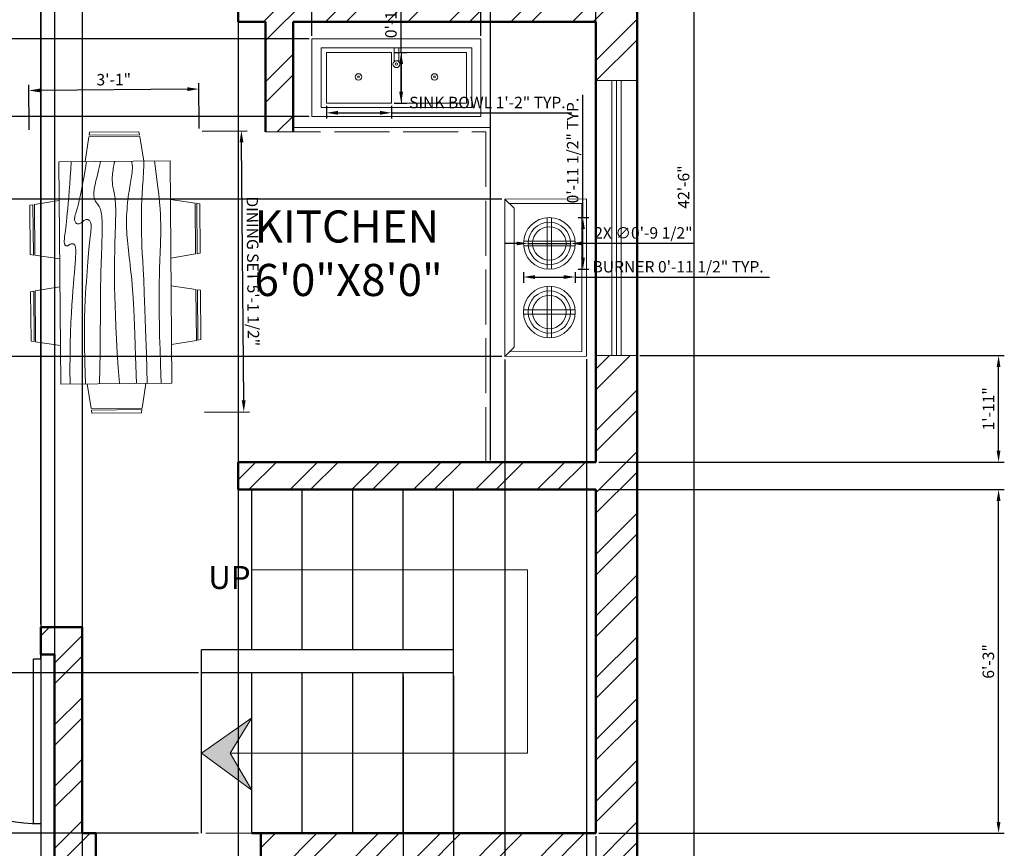
# Model space of a CAD drawing. Units: inches. Extents: x 1147 to 1568, y 1982 to 2559.
# Tile 3 of 4: x 1353 to 1568, y 2128 to 2309. Entities that reach past the tile are written whole.
import ezdxf

# ---------------------------------------------------------------- set-up
doc = ezdxf.new("R2010")
doc.units = ezdxf.units.IN
doc.linetypes.add('ACAD_ISO02W100', pattern=[15, 12, -3])
for name, color, linetype, lineweight in [('A-ANNO-DIMS', 2, 'Continuous', 18), ('A-ANNO-SYMB', 7, 'Continuous', 18), ('A-DOOR', 4, 'Continuous', 25), ('A-EQPM', 8, 'Continuous', 18), ('A-FLOR-CASE', 8, 'Continuous', 18), ('A-FLOR-CASE-HIDN', 8, 'ACAD_ISO02W100', 18), ('A-FLOR-FIXT', 8, 'Continuous', 18), ('A-FLOR-STRS', 7, 'Continuous', 25), ('A-WALL', 7, 'Continuous', 50), ('A-WALL-PATT', 252, 'Continuous', 13)]:
    doc.layers.add(name, color=color, linetype=linetype, lineweight=lineweight)
for name, color, linetype, lineweight, true_color in [('A-ANNO-TEXT', 244, 'Continuous', 18, 0x991b1e), ('A-AREA-IDEN', 244, 'Continuous', 25, 0x991b1e), ('A-FURN', 244, 'Continuous', 18, 0x991b1e), ('A-GLAZ', 177, 'Continuous', 18, 0x293189), ('A-WALL-OVHD', 244, 'ACAD_ISO02W100', 18, 0x991b1e)]:
    doc.layers.add(name, color=color, linetype=linetype, lineweight=lineweight, true_color=true_color)
doc.styles.get("Standard").update_dxf_attribs({"font": 'arial.ttf'})
doc.dimstyles.new('ISO-25', dxfattribs={"dimtxt": 2.5, "dimasz": 2.5, "dimexe": 1.25, "dimexo": 0.625, "dimtad": 1, "dimlunit": 3, "dimtxsty": 'Standard', "dimcen": 2.5, "dimadec": 0, "dimazin": 0, "dimtfac": 1, "dimtmove": 0, "dimatfit": 3, "dimfxl": 1, "dimarcsym": 0})

# ---------------------------------------------------------------- blocks, each defined once
blk = doc.blocks.new('*U3')
for p, q in [((-40, 0), (-40, 6)), ((0, 0), (0, 6))]:
    blk.add_line(p, q)
blk.add_lwpolyline([(0, 0), (0, -40), (-1.75, -40), (-1.75, 0)], close=True)
blk.add_arc((0, 0), 40, 180, 270)
blk = doc.blocks.new('Dining Set - 36 x 72 in.')
for p, q in [((-22.2343, 26.00059), (-23.4847, 17.99762)), ((-22.2304, 26), (-5.7608, 26)), ((-22, 27.5), (-22.1562, 26.50042)), ((-5.8416, 26.5), (-22.1534, 26.5)), ((-22, 27.5), (-6, 27.5)), ((-5.8437, 26.49966), (-6, 27.5)), ((-4.5152, 17.99762), (-5.7655, 25.99926)), ((5.7657, 26.00059), (4.5153, 17.99762)), ((5.7696, 26), (22.2392, 26)), ((6, 27.5), (5.8438, 26.50042)), ((22.1584, 26.5), (5.8466, 26.5)), ((6, 27.5), (22, 27.5)), ((22.1563, 26.49966), (22, 27.5)), ((23.4848, 17.99762), (22.2345, 25.99926)), ((36, 18), (-36, 18)), ((-36, 18), (-36, -18)), ((36, -18), (36, 18)), ((-45.5, 8), (-44.5004, 8.15617)), ((-45.5, 8), (-45.5, -8)), ((-44.5, -8.15843), (-44.5, 8.15338)), ((-44.0006, 8.23428), (-35.9976, 9.48474)), ((-44, 8.23041), (-44, -8.23915)), ((44.0006, 8.23428), (35.9976, 9.48474)), ((44, 8.23041), (44, -8.23915)), ((44.5, -8.15843), (44.5, 8.15338)), ((45.5, 8), (44.5005, 8.15617)), ((45.5, 8), (45.5, -8)), ((-44.4997, -8.15631), (-45.5, -8)), ((-35.9976, -9.48476), (-43.9993, -8.2345)), ((35.9976, -9.48476), (43.9993, -8.2345)), ((44.4997, -8.15631), (45.5, -8)), ((-36, -18), (36, -18)), ((-22.2343, -26.0006), (-23.4847, -17.99762)), ((-4.5152, -17.99762), (-5.7655, -25.99928)), ((5.7657, -26.0006), (4.5153, -17.99762)), ((23.4848, -17.99762), (22.2345, -25.99928)), ((-22.2304, -26), (-5.7608, -26)), ((-22, -27.5), (-22.1562, -26.50044)), ((-5.8416, -26.5), (-22.1534, -26.5)), ((-22, -27.5), (-6, -27.5)), ((-5.8437, -26.49967), (-6, -27.5)), ((5.7696, -26), (22.2392, -26)), ((6, -27.5), (5.8438, -26.50044)), ((22.1584, -26.5), (5.8466, -26.5)), ((6, -27.5), (22, -27.5)), ((22.1563, -26.49967), (22, -27.5))]:
    blk.add_line(p, q)
for points in [[(-36, 15), (-31.1772, 14.97754), (-26.8079, 14.91406), (-22.8538, 14.81543), (-19.276, 14.6875), (-16.0362, 14.53613), (-13.0957, 14.36718), (-10.4159, 14.18652), (-7.9583, 14), (-5.6904, 13.81315), (-3.6035, 13.63021), (-1.6954, 13.45508), (0.0365, 13.29166), (1.5945, 13.14388), (2.9811, 13.01562), (4.1988, 12.9108), (5.25, 12.83333), (6.1393, 12.78613), (6.8802, 12.76823), (7.4883, 12.77767), (7.9792, 12.8125), (8.3685, 12.87077), (8.6719, 12.95052), (8.9049, 13.0498), (9.0833, 13.16666), (9.2205, 13.29899), (9.3216, 13.44401), (9.3895, 13.59879), (9.4271, 13.76041), (9.4373, 13.92594), (9.4232, 14.09245), (9.3875, 14.257), (9.3333, 14.41666), (9.2638, 14.56917), (9.1836, 14.71484), (9.0975, 14.85465), (9.0104, 14.98958), (8.9272, 15.1206), (8.8529, 15.2487), (8.7922, 15.37483), (8.75, 15.5), (8.7305, 15.62467), (8.7344, 15.74739), (8.7617, 15.86621), (8.8125, 15.97916), (8.8867, 16.08431), (8.9844, 16.17968), (9.1055, 16.26334), (9.25, 16.33333), (9.4189, 16.38802), (9.6172, 16.42708), (9.8506, 16.45052), (10.125, 16.45833), (10.4463, 16.45052), (10.8203, 16.42708), (11.2529, 16.38802), (11.75, 16.33333), (12.3184, 16.26318), (12.9694, 16.17838), (13.7151, 16.07991), (14.5677, 15.96875), (15.5395, 15.84586), (16.6426, 15.71224), (17.8893, 15.56884), (19.2917, 15.41666), (20.859, 15.25667), (22.5879, 15.08984), (24.4721, 14.91715), (26.5052, 14.73958), (28.6809, 14.5581), (30.9929, 14.3737), (33.4347, 14.18733), (36, 14)], [(-36, 10), (-28.9766, 10.14274), (-23.1725, 10.20442), (-18.4241, 10.19775), (-14.5677, 10.13541), (-11.4399, 10.03011), (-8.877, 9.89453), (-6.7154, 9.74137), (-4.7917, 9.58333), (-2.9698, 9.43082), (-1.2246, 9.28515), (0.4415, 9.14534), (2.026, 9.01041), (3.5266, 8.87939), (4.9408, 8.7513), (6.266, 8.62516), (7.5, 8.5), (8.6411, 8.37549), (9.6914, 8.2539), (10.6538, 8.13818), (11.5312, 8.03125), (12.3267, 7.93603), (13.043, 7.85547), (13.6831, 7.79248), (14.25, 7.75), (14.7471, 7.7303), (15.1797, 7.73307), (15.5537, 7.75732), (15.875, 7.80208), (16.1494, 7.86637), (16.3828, 7.94922), (16.5811, 8.04964), (16.75, 8.16666), (16.8944, 8.29915), (17.0143, 8.44531), (17.1089, 8.60319), (17.1771, 8.77083), (17.218, 8.94629), (17.2305, 9.1276), (17.2137, 9.31282), (17.1667, 9.5), (17.0895, 9.6875), (16.987, 9.875), (16.8649, 10.0625), (16.7292, 10.25), (16.5856, 10.4375), (16.4401, 10.625), (16.2985, 10.8125), (16.1667, 11), (16.05, 11.18733), (15.9518, 11.3737), (15.8752, 11.5581), (15.8229, 11.73958), (15.798, 11.91715), (15.8034, 12.08984), (15.842, 12.25667), (15.9167, 12.41666), (16.0295, 12.56836), (16.1784, 12.70833), (16.3605, 12.83268), (16.5729, 12.9375), (16.8127, 13.01888), (17.0768, 13.07291), (17.3625, 13.0957), (17.6667, 13.08333), (17.9894, 13.03312), (18.3418, 12.94726), (18.7382, 12.82918), (19.1927, 12.68229), (19.7195, 12.51001), (20.3327, 12.31575), (21.0465, 12.10294), (21.875, 11.875), (22.8357, 11.63354), (23.959, 11.37304), (25.2786, 11.08618), (26.8282, 10.76562), (28.6414, 10.40405), (30.752, 9.99414), (33.1936, 9.52856), (36, 9)], [(-36, 5.5), (-30.7157, 5.3348), (-26.069, 5.20963), (-21.9946, 5.11767), (-18.4271, 5.05208), (-15.3009, 5.00602), (-12.5508, 4.97265), (-10.1112, 4.94515), (-7.9167, 4.91666), (-5.909, 4.88167), (-4.0586, 4.83984), (-2.3429, 4.79215), (-0.7396, 4.73958), (0.7739, 4.6831), (2.22, 4.6237), (3.6213, 4.56233), (5, 4.5), (6.373, 4.43782), (7.7344, 4.3776), (9.0723, 4.32129), (10.375, 4.27083), (11.6309, 4.22819), (12.8281, 4.19531), (13.9551, 4.17415), (15, 4.16666), (15.954, 4.17448), (16.819, 4.19791), (17.6001, 4.23698), (18.3021, 4.29166), (18.9299, 4.36198), (19.4883, 4.44791), (19.9823, 4.54948), (20.4167, 4.66666), (20.7969, 4.79899), (21.1302, 4.94401), (21.4245, 5.09879), (21.6875, 5.26041), (21.9271, 5.42594), (22.1511, 5.59245), (22.3672, 5.757), (22.5834, 5.91666), (22.8065, 6.06868), (23.0404, 6.21093), (23.2879, 6.34147), (23.5521, 6.45833), (23.8358, 6.55957), (24.142, 6.64323), (24.4735, 6.70735), (24.8334, 6.75), (25.2235, 6.76969), (25.642, 6.76692), (26.0858, 6.74267), (26.5521, 6.69791), (27.0379, 6.63362), (27.5404, 6.55078), (28.0565, 6.45036), (28.5834, 6.33333), (29.1242, 6.19987), (29.7071, 6.04687), (30.3661, 5.87044), (31.1354, 5.66666), (32.0493, 5.43164), (33.142, 5.16146), (34.4475, 4.85221), (36, 4.5)], [(-36, -1), (-30.7915, -0.6591), (-26.0195, -0.38216), (-21.6519, -0.16284), (-17.6563, 0.00521), (-14.0005, 0.12833), (-10.6523, 0.21289), (-7.5796, 0.26522), (-4.75, 0.29166), (-2.134, 0.29793), (0.2878, 0.28711), (2.5317, 0.26163), (4.6146, 0.22396), (6.5529, 0.17651), (8.3633, 0.12174), (10.0623, 0.06209), (11.6667, 0), (13.1899, -0.06201), (14.6341, -0.1211), (15.9982, -0.17432), (17.2813, -0.21875), (18.4823, -0.25147), (19.6003, -0.26953), (20.6343, -0.27002), (21.5834, -0.25), (22.4481, -0.20768), (23.2357, -0.14584), (23.9549, -0.06836), (24.6146, 0.02083), (25.2235, 0.11784), (25.7904, 0.21875), (26.3241, 0.31966), (26.8334, 0.41666), (27.3265, 0.50618), (27.8099, 0.58593), (28.2894, 0.65397), (28.7709, 0.70833), (29.2601, 0.74707), (29.763, 0.76823), (30.2855, 0.76985), (30.8334, 0.75), (31.4088, 0.70784), (31.9994, 0.64713), (32.589, 0.57275), (33.1615, 0.48958), (33.7008, 0.4025), (34.1908, 0.3164), (34.6153, 0.23616), (34.9584, 0.16666), (35.2099, 0.11165), (35.3848, 0.07031), (35.504, 0.04069), (35.5886, 0.02083), (35.6594, 0.00879), (35.7377, 0.0026), (35.8442, 0.00032), (36, 0)], [(-36, -6.5), (-27.1843, -6.31267), (-20.084, -6.1263), (-14.469, -5.9419), (-10.1094, -5.76042), (-6.7752, -5.58285), (-4.2363, -5.41016), (-2.2629, -5.24333), (-0.625, -5.08334), (0.8708, -4.93099), (2.2715, -4.78646), (3.5872, -4.64974), (4.8281, -4.52084), (6.0046, -4.39974), (7.127, -4.28646), (8.2053, -4.18099), (9.25, -4.08334), (10.2705, -3.99382), (11.2734, -3.91407), (12.2647, -3.84603), (13.25, -3.79167), (14.2354, -3.75293), (15.2266, -3.73177), (16.2295, -3.73015), (17.25, -3.75), (18.2912, -3.79248), (19.3451, -3.85547), (20.4009, -3.93604), (21.4479, -4.03125), (22.4754, -4.13819), (23.4727, -4.25391), (24.4289, -4.37549), (25.3334, -4.5), (26.1785, -4.62492), (26.9694, -4.74935), (27.7145, -4.87281), (28.4219, -4.99479), (29.1, -5.11483), (29.7572, -5.23242), (30.4016, -5.34709), (31.0417, -5.45834), (31.6837, -5.56437), (32.3262, -5.65821), (32.9658, -5.73153), (33.599, -5.77604), (34.2224, -5.78345), (34.8327, -5.74545), (35.4264, -5.65373), (36, -5.5)], [(-36, -10), (-26.4022, -9.81299), (-18.4675, -9.62891), (-11.9839, -9.45069), (-6.7396, -9.28125), (-2.5226, -9.12354), (0.8789, -8.98047), (3.6769, -8.85498), (6.0833, -8.75), (8.2767, -8.66765), (10.3021, -8.60677), (12.1712, -8.56543), (13.8958, -8.54167), (15.4876, -8.53353), (16.9583, -8.53907), (18.3197, -8.55632), (19.5834, -8.58334), (20.7616, -8.61841), (21.8685, -8.66081), (22.9188, -8.71004), (23.9271, -8.76563), (24.9081, -8.82707), (25.8763, -8.89388), (26.8465, -8.96558), (27.8334, -9.04167), (28.8474, -9.12118), (29.8828, -9.20117), (30.93, -9.27824), (31.9792, -9.34896), (33.0205, -9.40991), (34.0443, -9.45768), (35.0407, -9.48885), (36, -9.5)], [(-36, -14.5), (-30.0881, -14.33513), (-25.0332, -14.21224), (-20.7312, -14.12647), (-17.0781, -14.07292), (-13.97, -14.04671), (-11.3027, -14.04297), (-8.9724, -14.05681), (-6.875, -14.08334), (-4.9224, -14.11833), (-3.0905, -14.16016), (-1.3709, -14.20785), (0.2448, -14.26042), (1.7647, -14.3169), (3.1973, -14.3763), (4.5507, -14.43767), (5.8333, -14.5), (7.0554, -14.5621), (8.235, -14.62175), (9.3922, -14.67652), (10.5469, -14.72396), (11.7192, -14.76164), (12.929, -14.78711), (14.1965, -14.79794), (15.5417, -14.79167), (16.9933, -14.76424), (18.6152, -14.70508), (20.4804, -14.60197), (22.6615, -14.44271), (25.2312, -14.21509), (28.2624, -13.9069), (31.8277, -13.50594), (36, -13)]]:
    blk.add_lwpolyline(points)
blk = doc.blocks.new('*D13')
at = {"layer": 'A-ANNO-DIMS', "color": 0, "lineweight": -2, "transparency": 16777216}
for p, q in [((1488.23, 2527.7), (1501.22, 2527.7)), ((1499.97, 2525.2), (1499.97, 2020.2)), ((1488.23, 2017.7), (1501.22, 2017.7))]:
    blk.add_line(p, q, dxfattribs=at)
at = {"layer": 'A-ANNO-DIMS', "color": 0, "transparency": 16777216}
for points in [[(1499.56, 2525.2), (1500.39, 2525.2), (1499.97, 2527.7)], [(1499.56, 2020.2), (1500.39, 2020.2), (1499.97, 2017.7)]]:
    blk.add_solid(points, dxfattribs=at)
at = {"layer": 'Defpoints', "color": 0, "transparency": 16777216}
for p in [(1487.61, 2527.7), (1487.61, 2017.7), (1499.97, 2017.7)]:
    blk.add_point(p, dxfattribs=at)
at = {"layer": 'A-ANNO-DIMS', "color": 0, "transparency": 16777216, "insert": (1498.07, 2272.7), "char_height": 2.5, "attachment_point": 5, "rotation": 90}
blk.add_mtext('42\'-6"', dxfattribs=at)
blk = doc.blocks.new('WIN-GLAZ-60IN')
for p, q in [((0, 60), (0, 0)), ((1, 60), (1, 0)), ((2, 60), (2, 0))]:
    blk.add_line(p, q)
blk = doc.blocks.new('COOKTOP-BURNER')
for p, q in [((5.14, 11.27), (5.14, 0)), ((6.14, 11.27), (6.14, 0)), ((0, 6.14), (11.27, 6.14)), ((0, 5.14), (11.27, 5.14))]:
    blk.add_line(p, q)
for radius in [5.64, 4.64, 3.64]:
    blk.add_circle((5.64, 5.64), radius)
blk = doc.blocks.new('SINK-BOWL-WITH-DRAIN')
blk.add_lwpolyline([(0, 11.03), (14.13, 11.03), (14.13, 0), (0, 0)], close=True)
for radius in [0.702, 0.202]:
    blk.add_circle((6.95, 5.7), radius)
blk = doc.blocks.new('*D29')
at = {"layer": 'A-ANNO-DIMS', "color": 0, "lineweight": -2, "transparency": 16777216}
for p, q in [((1462.84, 2254.12), (1462.84, 2251.81)), ((1474.11, 2254.12), (1474.11, 2251.81)), ((1465.34, 2253.06), (1471.61, 2253.06)), ((1474.11, 2253.06), (1516.47, 2253.06))]:
    blk.add_line(p, q, dxfattribs=at)
at = {"layer": 'A-ANNO-DIMS', "color": 0, "transparency": 16777216}
for points in [[(1465.34, 2253.47), (1465.34, 2252.64), (1462.84, 2253.06)], [(1471.61, 2253.47), (1471.61, 2252.64), (1474.11, 2253.06)]]:
    blk.add_solid(points, dxfattribs=at)
at = {"layer": 'Defpoints', "color": 0, "transparency": 16777216}
for p in [(1462.84, 2254.75), (1474.11, 2254.75), (1474.11, 2253.06)]:
    blk.add_point(p, dxfattribs=at)
at = {"layer": 'A-ANNO-DIMS', "color": 0, "transparency": 16777216, "insert": (1496.54, 2254.98), "char_height": 2.5, "attachment_point": 5}
blk.add_mtext('BURNER 0\'-11 1/2" TYP.', dxfattribs=at)
blk = doc.blocks.new('*D30')
at = {"layer": 'A-ANNO-DIMS', "color": 0, "lineweight": -2, "transparency": 16777216}
for p, q in [((1475.8, 2266.02), (1475.8, 2292.78)), ((1474.73, 2266.02), (1477.05, 2266.02)), ((1475.8, 2257.25), (1475.8, 2263.52)), ((1474.73, 2254.75), (1477.05, 2254.75))]:
    blk.add_line(p, q, dxfattribs=at)
at = {"layer": 'A-ANNO-DIMS', "color": 0, "transparency": 16777216}
for points in [[(1475.38, 2263.52), (1476.22, 2263.52), (1475.8, 2266.02)], [(1475.38, 2257.25), (1476.22, 2257.25), (1475.8, 2254.75)]]:
    blk.add_solid(points, dxfattribs=at)
at = {"layer": 'Defpoints', "color": 0, "transparency": 16777216}
for p in [(1474.11, 2266.02), (1475.8, 2266.02), (1474.11, 2254.75)]:
    blk.add_point(p, dxfattribs=at)
at = {"layer": 'A-ANNO-DIMS', "color": 0, "transparency": 16777216, "insert": (1473.88, 2280.65), "char_height": 2.5, "attachment_point": 5, "rotation": 90}
blk.add_mtext('0\'-11 1/2" TYP.', dxfattribs=at)
blk = doc.blocks.new('*D31')
at = {"layer": 'A-ANNO-DIMS', "color": 0, "lineweight": -2, "transparency": 16777216}
for p, q in [((1419.91, 2290.39), (1419.91, 2287.64)), ((1434.04, 2290.39), (1434.04, 2287.64)), ((1422.41, 2288.89), (1431.54, 2288.89)), ((1434.04, 2288.89), (1473.4, 2288.89))]:
    blk.add_line(p, q, dxfattribs=at)
at = {"layer": 'A-ANNO-DIMS', "color": 0, "transparency": 16777216}
for points in [[(1422.41, 2289.31), (1422.41, 2288.47), (1419.91, 2288.89)], [(1431.54, 2289.31), (1431.54, 2288.47), (1434.04, 2288.89)]]:
    blk.add_solid(points, dxfattribs=at)
at = {"layer": 'Defpoints', "color": 0, "transparency": 16777216}
for p in [(1419.91, 2291.01), (1434.04, 2291.01), (1434.04, 2288.89)]:
    blk.add_point(p, dxfattribs=at)
at = {"layer": 'A-ANNO-DIMS', "color": 0, "transparency": 16777216, "insert": (1454.97, 2290.81), "char_height": 2.5, "attachment_point": 5}
blk.add_mtext('SINK BOWL 1\'-2" TYP.', dxfattribs=at)
blk = doc.blocks.new('*D32')
at = {"layer": 'A-ANNO-DIMS', "color": 0, "lineweight": -2, "transparency": 16777216}
for p, q in [((1436.16, 2302.04), (1436.16, 2322.97)), ((1434.67, 2302.04), (1437.41, 2302.04)), ((1436.16, 2293.51), (1436.16, 2299.54)), ((1434.67, 2291.01), (1437.41, 2291.01))]:
    blk.add_line(p, q, dxfattribs=at)
at = {"layer": 'A-ANNO-DIMS', "color": 0, "transparency": 16777216}
for points in [[(1435.75, 2299.54), (1436.58, 2299.54), (1436.16, 2302.04)], [(1435.75, 2293.51), (1436.58, 2293.51), (1436.16, 2291.01)]]:
    blk.add_solid(points, dxfattribs=at)
at = {"layer": 'Defpoints', "color": 0, "transparency": 16777216}
for p in [(1434.04, 2302.04), (1436.16, 2302.04), (1434.04, 2291.01)]:
    blk.add_point(p, dxfattribs=at)
at = {"layer": 'A-ANNO-DIMS', "color": 0, "transparency": 16777216, "insert": (1434.26, 2313.75), "char_height": 2.5, "attachment_point": 5, "rotation": 90}
blk.add_mtext('0\'-11" TYP.', dxfattribs=at)
blk = doc.blocks.new('*D37')
at = {"layer": 'A-ANNO-DIMS', "color": 0, "lineweight": -2, "transparency": 16777216}
for p, q in [((1392.77, 2284.88), (1402.59, 2284.96)), ((1401.84, 2226.14), (1401.36, 2282.45)), ((1393.29, 2223.57), (1403.11, 2223.65))]:
    blk.add_line(p, q, dxfattribs=at)
at = {"layer": 'A-ANNO-DIMS', "color": 0, "transparency": 16777216}
for points in [[(1401.78, 2282.45), (1400.94, 2282.44), (1401.34, 2284.95)], [(1402.26, 2226.15), (1401.42, 2226.14), (1401.86, 2223.64)]]:
    blk.add_solid(points, dxfattribs=at)
at = {"layer": 'Defpoints', "color": 0, "transparency": 16777216}
for p in [(1392.14, 2284.87), (1401.34, 2284.95), (1392.67, 2223.57)]:
    blk.add_point(p, dxfattribs=at)
at = {"layer": 'A-ANNO-DIMS', "color": 0, "transparency": 16777216, "insert": (1403.52, 2254.31), "char_height": 2.5, "attachment_point": 5, "rotation": 270.4889}
blk.add_mtext('DINING SET 5\'-1 1/2"', dxfattribs=at)
blk = doc.blocks.new('*D38')
at = {"layer": 'A-ANNO-DIMS', "color": 0, "lineweight": -2, "transparency": 16777216}
for p, q in [((1355.09, 2285.18), (1355, 2295)), ((1392.14, 2285.49), (1392.05, 2295.32)), ((1389.56, 2294.04), (1357.51, 2293.77))]:
    blk.add_line(p, q, dxfattribs=at)
at = {"layer": 'A-ANNO-DIMS', "color": 0, "transparency": 16777216}
for points in [[(1357.51, 2294.19), (1357.52, 2293.35), (1355.01, 2293.75)], [(1389.56, 2294.46), (1389.57, 2293.63), (1392.06, 2294.07)]]:
    blk.add_solid(points, dxfattribs=at)
at = {"layer": 'Defpoints', "color": 0, "transparency": 16777216}
for p in [(1355.01, 2293.75), (1355.09, 2284.55), (1392.14, 2284.87)]:
    blk.add_point(p, dxfattribs=at)
at = {"layer": 'A-ANNO-DIMS', "color": 0, "transparency": 16777216, "insert": (1373.52, 2295.81), "char_height": 2.5, "attachment_point": 5, "rotation": 0.4889}
blk.add_mtext('3\'-1"', dxfattribs=at)
blk = doc.blocks.new('*D43')
at = {"layer": 'A-ANNO-DIMS', "color": 0, "lineweight": -2, "transparency": 16777216}
for p, q in [((1327.61, 2368.08), (1327.61, 1981.52)), ((1357.61, 2368.08), (1357.61, 1981.52)), ((1330.11, 1982.77), (1355.11, 1982.77))]:
    blk.add_line(p, q, dxfattribs=at)
at = {"layer": 'A-ANNO-DIMS', "color": 0, "transparency": 16777216}
for points in [[(1330.11, 1983.19), (1330.11, 1982.35), (1327.61, 1982.77)], [(1355.11, 1983.19), (1355.11, 1982.35), (1357.61, 1982.77)]]:
    blk.add_solid(points, dxfattribs=at)
at = {"layer": 'Defpoints', "color": 0, "transparency": 16777216}
for p in [(1327.61, 2368.7), (1357.61, 2368.7), (1357.61, 1982.77)]:
    blk.add_point(p, dxfattribs=at)
at = {"layer": 'A-ANNO-DIMS', "color": 0, "transparency": 16777216, "insert": (1342.61, 1984.67), "char_height": 2.5, "attachment_point": 5}
blk.add_mtext('2\'-6"', dxfattribs=at)
blk = doc.blocks.new('*D45')
at = {"layer": 'A-ANNO-DIMS', "color": 0, "lineweight": -2, "transparency": 16777216}
for p, q in [((1321.61, 2177.33), (1321.61, 2556.75)), ((1357.61, 2177.33), (1357.61, 2556.75)), ((1324.11, 2555.5), (1355.11, 2555.5))]:
    blk.add_line(p, q, dxfattribs=at)
at = {"layer": 'A-ANNO-DIMS', "color": 0, "transparency": 16777216}
for points in [[(1324.11, 2555.92), (1324.11, 2555.09), (1321.61, 2555.5)], [(1355.11, 2555.92), (1355.11, 2555.09), (1357.61, 2555.5)]]:
    blk.add_solid(points, dxfattribs=at)
at = {"layer": 'Defpoints', "color": 0, "transparency": 16777216}
for p in [(1357.61, 2555.5), (1321.61, 2176.7), (1357.61, 2176.7)]:
    blk.add_point(p, dxfattribs=at)
at = {"layer": 'A-ANNO-DIMS', "color": 0, "transparency": 16777216, "insert": (1339.61, 2557.41), "char_height": 2.5, "attachment_point": 5}
blk.add_mtext('3\'-0"', dxfattribs=at)
blk = doc.blocks.new('*D47')
at = {"layer": 'A-ANNO-DIMS', "color": 0, "lineweight": -2, "transparency": 16777216}
for p, q in [((1436.61, 2166.08), (1436.61, 1981.52)), ((1447.61, 2166.08), (1447.61, 1981.52)), ((1445.11, 1982.77), (1439.11, 1982.77))]:
    blk.add_line(p, q, dxfattribs=at)
at = {"layer": 'A-ANNO-DIMS', "color": 0, "transparency": 16777216}
for points in [[(1439.11, 1983.19), (1439.11, 1982.35), (1436.61, 1982.77)], [(1445.11, 1983.19), (1445.11, 1982.35), (1447.61, 1982.77)]]:
    blk.add_solid(points, dxfattribs=at)
at = {"layer": 'Defpoints', "color": 0, "transparency": 16777216}
for p in [(1436.61, 2166.7), (1447.61, 2166.7), (1436.61, 1982.77)]:
    blk.add_point(p, dxfattribs=at)
at = {"layer": 'A-ANNO-DIMS', "color": 0, "transparency": 16777216, "insert": (1442.11, 1984.67), "char_height": 2.5, "attachment_point": 5}
blk.add_mtext('0\'-11"', dxfattribs=at)
blk = doc.blocks.new('*D48')
at = {"layer": 'A-ANNO-DIMS', "color": 0, "lineweight": -2, "transparency": 16777216}
for p, q in [((1391.98, 2166.7), (1151.56, 2166.7)), ((1152.81, 2134.2), (1152.81, 2164.2)), ((1391.98, 2131.7), (1151.56, 2131.7))]:
    blk.add_line(p, q, dxfattribs=at)
at = {"layer": 'A-ANNO-DIMS', "color": 0, "transparency": 16777216}
for points in [[(1152.39, 2164.2), (1153.22, 2164.2), (1152.81, 2166.7)], [(1152.39, 2134.2), (1153.22, 2134.2), (1152.81, 2131.7)]]:
    blk.add_solid(points, dxfattribs=at)
at = {"layer": 'Defpoints', "color": 0, "transparency": 16777216}
for p in [(1152.81, 2166.7), (1392.61, 2166.7), (1392.61, 2131.7)]:
    blk.add_point(p, dxfattribs=at)
at = {"layer": 'A-ANNO-DIMS', "color": 0, "transparency": 16777216, "insert": (1150.93, 2149.2), "char_height": 2.5, "attachment_point": 5, "rotation": 90}
blk.add_mtext('2\'-11"', dxfattribs=at)
blk = doc.blocks.new('*D49')
at = {"layer": 'A-ANNO-DIMS', "color": 0, "lineweight": -2, "transparency": 16777216}
for p, q in [((1447.61, 2131.08), (1447.61, 1981.52)), ((1478.61, 2131.08), (1478.61, 1981.52)), ((1450.11, 1982.77), (1476.11, 1982.77))]:
    blk.add_line(p, q, dxfattribs=at)
at = {"layer": 'A-ANNO-DIMS', "color": 0, "transparency": 16777216}
for points in [[(1450.11, 1983.19), (1450.11, 1982.35), (1447.61, 1982.77)], [(1476.11, 1983.19), (1476.11, 1982.35), (1478.61, 1982.77)]]:
    blk.add_solid(points, dxfattribs=at)
at = {"layer": 'Defpoints', "color": 0, "transparency": 16777216}
for p in [(1447.61, 2131.7), (1478.61, 2131.7), (1478.61, 1982.77)]:
    blk.add_point(p, dxfattribs=at)
at = {"layer": 'A-ANNO-DIMS', "color": 0, "transparency": 16777216, "insert": (1463.11, 1984.65), "char_height": 2.5, "attachment_point": 5}
blk.add_mtext('2\'-7"', dxfattribs=at)
blk = doc.blocks.new('*D50')
at = {"layer": 'A-ANNO-DIMS', "color": 0, "lineweight": -2, "transparency": 16777216}
for p, q in [((1479.23, 2206.7), (1567.66, 2206.7)), ((1566.41, 2134.2), (1566.41, 2204.2)), ((1479.23, 2131.7), (1567.66, 2131.7))]:
    blk.add_line(p, q, dxfattribs=at)
at = {"layer": 'A-ANNO-DIMS', "color": 0, "transparency": 16777216}
for points in [[(1565.99, 2204.2), (1566.82, 2204.2), (1566.41, 2206.7)], [(1565.99, 2134.2), (1566.82, 2134.2), (1566.41, 2131.7)]]:
    blk.add_solid(points, dxfattribs=at)
at = {"layer": 'Defpoints', "color": 0, "transparency": 16777216}
for p in [(1478.61, 2206.7), (1566.41, 2206.7), (1478.61, 2131.7)]:
    blk.add_point(p, dxfattribs=at)
at = {"layer": 'A-ANNO-DIMS', "color": 0, "transparency": 16777216, "insert": (1564.5, 2169.2), "char_height": 2.5, "attachment_point": 5, "rotation": 90}
blk.add_mtext('6\'-3"', dxfattribs=at)
blk = doc.blocks.new('*D51')
at = {"layer": 'A-ANNO-DIMS', "color": 0, "lineweight": -2, "transparency": 16777216}
for p, q in [((1360.61, 2518.08), (1360.61, 1981.52)), ((1366.61, 2518.08), (1366.61, 1981.52)), ((1358.11, 1982.77), (1355.61, 1982.77)), ((1360.61, 1982.77), (1366.61, 1982.77)), ((1369.11, 1982.77), (1379.5, 1982.77))]:
    blk.add_line(p, q, dxfattribs=at)
at = {"layer": 'A-ANNO-DIMS', "color": 0, "transparency": 16777216}
for points in [[(1358.11, 1983.19), (1358.11, 1982.35), (1360.61, 1982.77)], [(1369.11, 1983.19), (1369.11, 1982.35), (1366.61, 1982.77)]]:
    blk.add_solid(points, dxfattribs=at)
at = {"layer": 'Defpoints', "color": 0, "transparency": 16777216}
for p in [(1360.61, 2518.7), (1366.61, 2518.7), (1366.61, 1982.77)]:
    blk.add_point(p, dxfattribs=at)
at = {"layer": 'A-ANNO-DIMS', "color": 0, "transparency": 16777216, "insert": (1375.55, 1984.67), "char_height": 2.5, "attachment_point": 5}
blk.add_mtext('0\'-6"', dxfattribs=at)
blk = doc.blocks.new('*D60')
at = {"layer": 'A-ANNO-DIMS', "color": 0, "lineweight": -2, "transparency": 16777216}
for p, q in [((1488.23, 2235.92), (1567.66, 2235.92)), ((1566.41, 2215.2), (1566.41, 2233.42)), ((1479.23, 2212.7), (1567.66, 2212.7))]:
    blk.add_line(p, q, dxfattribs=at)
at = {"layer": 'A-ANNO-DIMS', "color": 0, "transparency": 16777216}
for points in [[(1565.99, 2233.42), (1566.82, 2233.42), (1566.41, 2235.92)], [(1565.99, 2215.2), (1566.82, 2215.2), (1566.41, 2212.7)]]:
    blk.add_solid(points, dxfattribs=at)
at = {"layer": 'Defpoints', "color": 0, "transparency": 16777216}
for p in [(1487.61, 2235.92), (1566.41, 2235.92), (1478.61, 2212.7)]:
    blk.add_point(p, dxfattribs=at)
at = {"layer": 'A-ANNO-DIMS', "color": 0, "transparency": 16777216, "insert": (1564.53, 2224.31), "char_height": 2.5, "attachment_point": 5, "rotation": 90}
blk.add_mtext('1\'-11"', dxfattribs=at)
blk = doc.blocks.new('*D61')
at = {"layer": 'A-ANNO-DIMS', "color": 0, "lineweight": -2, "transparency": 16777216}
for p, q in [((1455.61, 2213.33), (1455.61, 2556.75)), ((1478.61, 2213.33), (1478.61, 2556.75)), ((1458.11, 2555.5), (1476.11, 2555.5))]:
    blk.add_line(p, q, dxfattribs=at)
at = {"layer": 'A-ANNO-DIMS', "color": 0, "transparency": 16777216}
for points in [[(1458.11, 2555.92), (1458.11, 2555.09), (1455.61, 2555.5)], [(1476.11, 2555.92), (1476.11, 2555.09), (1478.61, 2555.5)]]:
    blk.add_solid(points, dxfattribs=at)
at = {"layer": 'Defpoints', "color": 0, "transparency": 16777216}
for p in [(1478.61, 2555.5), (1455.61, 2212.7), (1478.61, 2212.7)]:
    blk.add_point(p, dxfattribs=at)
at = {"layer": 'A-ANNO-DIMS', "color": 0, "transparency": 16777216, "insert": (1467.11, 2557.38), "char_height": 2.5, "attachment_point": 5}
blk.add_mtext('1\'-11"', dxfattribs=at)
blk = doc.blocks.new('*D62')
at = {"layer": 'A-ANNO-DIMS', "color": 0, "lineweight": -2, "transparency": 16777216}
for p, q in [((1324.61, 2335.08), (1324.61, 1981.52)), ((1400.61, 2335.08), (1400.61, 1981.52)), ((1327.11, 1982.77), (1398.11, 1982.77))]:
    blk.add_line(p, q, dxfattribs=at)
at = {"layer": 'A-ANNO-DIMS', "color": 0, "transparency": 16777216}
for points in [[(1327.11, 1983.19), (1327.11, 1982.35), (1324.61, 1982.77)], [(1398.11, 1983.19), (1398.11, 1982.35), (1400.61, 1982.77)]]:
    blk.add_solid(points, dxfattribs=at)
at = {"layer": 'Defpoints', "color": 0, "transparency": 16777216}
for p in [(1324.61, 2335.7), (1400.61, 2335.7), (1400.61, 1982.77)]:
    blk.add_point(p, dxfattribs=at)
at = {"layer": 'A-ANNO-DIMS', "color": 0, "transparency": 16777216, "insert": (1362.61, 1984.67), "char_height": 2.5, "attachment_point": 5}
blk.add_mtext('6\'-4"', dxfattribs=at)
blk = doc.blocks.new('*D65')
at = {"layer": 'A-ANNO-DIMS', "color": 0, "lineweight": -2, "transparency": 16777216}
for p, q in [((1458.78, 2235.1), (1458.78, 1981.52)), ((1476.55, 2235.16), (1476.55, 1981.52)), ((1461.28, 1982.77), (1474.05, 1982.77))]:
    blk.add_line(p, q, dxfattribs=at)
at = {"layer": 'A-ANNO-DIMS', "color": 0, "transparency": 16777216}
for points in [[(1461.28, 1983.19), (1461.28, 1982.35), (1458.78, 1982.77)], [(1474.05, 1983.19), (1474.05, 1982.35), (1476.55, 1982.77)]]:
    blk.add_solid(points, dxfattribs=at)
at = {"layer": 'Defpoints', "color": 0, "transparency": 16777216}
for p in [(1458.78, 2235.73), (1476.55, 2235.78), (1476.55, 1982.77)]:
    blk.add_point(p, dxfattribs=at)
at = {"layer": 'A-ANNO-DIMS', "color": 0, "transparency": 16777216, "insert": (1467.66, 1984.67), "char_height": 2.5, "attachment_point": 5}
blk.add_mtext('1\'-6"', dxfattribs=at)
blk = doc.blocks.new('*D66')
at = {"layer": 'A-ANNO-DIMS', "color": 0, "lineweight": -2, "transparency": 16777216}
for p, q in [((1458.15, 2270.07), (1151.56, 2270.07)), ((1152.81, 2238.23), (1152.81, 2267.57)), ((1458.15, 2235.73), (1151.56, 2235.73))]:
    blk.add_line(p, q, dxfattribs=at)
at = {"layer": 'A-ANNO-DIMS', "color": 0, "transparency": 16777216}
for points in [[(1152.39, 2267.57), (1153.22, 2267.57), (1152.81, 2270.07)], [(1152.39, 2238.23), (1153.22, 2238.23), (1152.81, 2235.73)]]:
    blk.add_solid(points, dxfattribs=at)
at = {"layer": 'Defpoints', "color": 0, "transparency": 16777216}
for p in [(1152.81, 2270.07), (1458.78, 2270.07), (1458.78, 2235.73)]:
    blk.add_point(p, dxfattribs=at)
at = {"layer": 'A-ANNO-DIMS', "color": 0, "transparency": 16777216, "insert": (1150.89, 2252.9), "char_height": 2.5, "attachment_point": 5, "rotation": 90}
blk.add_mtext('2\'-10 1/2"', dxfattribs=at)
blk = doc.blocks.new('*D67')
at = {"layer": 'A-ANNO-DIMS', "color": 0, "lineweight": -2, "transparency": 16777216}
for p, q in [((1416.72, 2305.68), (1416.72, 2556.75)), ((1453.56, 2305.68), (1453.56, 2556.75)), ((1419.22, 2555.5), (1451.06, 2555.5))]:
    blk.add_line(p, q, dxfattribs=at)
at = {"layer": 'A-ANNO-DIMS', "color": 0, "transparency": 16777216}
for points in [[(1419.22, 2555.92), (1419.22, 2555.09), (1416.72, 2555.5)], [(1451.06, 2555.92), (1451.06, 2555.09), (1453.56, 2555.5)]]:
    blk.add_solid(points, dxfattribs=at)
at = {"layer": 'Defpoints', "color": 0, "transparency": 16777216}
for p in [(1453.56, 2555.5), (1416.72, 2305.06), (1453.56, 2305.06)]:
    blk.add_point(p, dxfattribs=at)
at = {"layer": 'A-ANNO-DIMS', "color": 0, "transparency": 16777216, "insert": (1435.14, 2557.41), "char_height": 2.5, "attachment_point": 5}
blk.add_mtext('3\'-1"', dxfattribs=at)
blk = doc.blocks.new('*D68')
at = {"layer": 'A-ANNO-DIMS', "color": 0, "lineweight": -2, "transparency": 16777216}
for p, q in [((1416.1, 2305.06), (1151.56, 2305.06)), ((1152.81, 2302.56), (1152.81, 2290.56)), ((1416.1, 2288.06), (1151.56, 2288.06))]:
    blk.add_line(p, q, dxfattribs=at)
at = {"layer": 'A-ANNO-DIMS', "color": 0, "transparency": 16777216}
for points in [[(1152.39, 2302.56), (1153.22, 2302.56), (1152.81, 2305.06)], [(1152.39, 2290.56), (1153.22, 2290.56), (1152.81, 2288.06)]]:
    blk.add_solid(points, dxfattribs=at)
at = {"layer": 'Defpoints', "color": 0, "transparency": 16777216}
for p in [(1416.72, 2305.06), (1152.81, 2288.06), (1416.72, 2288.06)]:
    blk.add_point(p, dxfattribs=at)
at = {"layer": 'A-ANNO-DIMS', "color": 0, "transparency": 16777216, "insert": (1150.91, 2296.56), "char_height": 2.5, "attachment_point": 5, "rotation": 90}
blk.add_mtext('1\'-5"', dxfattribs=at)
blk = doc.blocks.new('*D72')
at = {"layer": 'A-ANNO-DIMS', "color": 0, "lineweight": -2, "transparency": 16777216}
for p, q in [((1461.34, 2260.39), (1458.84, 2260.39)), ((1463.84, 2260.39), (1473.11, 2260.39)), ((1499.83, 2260.38), (1475.61, 2260.38))]:
    blk.add_line(p, q, dxfattribs=at)
at = {"layer": 'A-ANNO-DIMS', "color": 0, "transparency": 16777216}
for points in [[(1461.34, 2260.8), (1461.34, 2259.97), (1463.84, 2260.39)], [(1475.61, 2260.8), (1475.61, 2259.97), (1473.11, 2260.39)]]:
    blk.add_solid(points, dxfattribs=at)
at = {"layer": 'Defpoints', "color": 0, "transparency": 16777216}
for p in [(1463.84, 2260.39), (1473.11, 2260.39)]:
    blk.add_point(p, dxfattribs=at)
at = {"layer": 'A-ANNO-DIMS', "color": 0, "transparency": 16777216, "insert": (1488.97, 2262.36), "char_height": 2.5, "attachment_point": 5, "rotation": 359.9973}
blk.add_mtext('2X ∅0\'-9 1/2"', dxfattribs=at)

msp = doc.modelspace()

# ---------------------------------------------------------------- hatches: boundary and pattern name
at = {"layer": 'A-ANNO-SYMB'}
h = msp.add_hatch(color=256, dxfattribs=at)
h.dxf.hatch_style = 1
h.paths.add_polyline_path([(1403.607, 2156.907), (1392.607, 2149.204), (1403.607, 2141.143), (1398.928, 2149.204)])
at = {"layer": 'A-WALL-PATT'}
h = msp.add_hatch(dxfattribs=at)
h.set_pattern_fill('ANSI32', color=256)
h.paths.add_polyline_path([(1240.607, 2518.704), (1268.63, 2518.704), (1268.63, 2527.704), (1231.607, 2527.704), (1231.607, 2348.295), (1240.607, 2348.295), (1240.607, 2368.704), (1318.607, 2368.704), (1318.607, 2365.704), (1324.607, 2365.704), (1324.607, 2368.704), (1327.607, 2368.704), (1327.607, 2374.704), (1240.607, 2374.704)])
h.paths.add_polyline_path([(1324.607, 2335.704), (1318.607, 2335.704), (1318.607, 2314.704), (1240.607, 2314.704), (1240.607, 2324.295), (1231.607, 2324.295), (1231.607, 2247.419), (1240.607, 2247.419), (1240.607, 2308.704), (1324.607, 2308.704)])
h.paths.add_polyline_path([(1487.607, 2527.704), (1464.679, 2527.704), (1464.679, 2518.704), (1478.607, 2518.704), (1478.607, 2374.704), (1399.607, 2374.704), (1399.607, 2368.704), (1400.607, 2368.704), (1400.607, 2365.704), (1406.607, 2365.704), (1406.607, 2368.704), (1478.607, 2368.704), (1478.607, 2343.549), (1487.607, 2343.549)])
h.paths.add_polyline_path([(1366.607, 2518.704), (1398.679, 2518.704), (1398.679, 2527.704), (1334.63, 2527.704), (1334.63, 2518.704), (1360.607, 2518.704), (1360.607, 2374.704), (1357.607, 2374.704), (1357.607, 2368.704), (1369.607, 2368.704), (1369.607, 2374.704), (1366.607, 2374.704)])
h.paths.add_polyline_path([(1487.607, 2319.549), (1478.607, 2319.549), (1478.607, 2314.704), (1406.607, 2314.704), (1406.607, 2335.704), (1400.607, 2335.704), (1400.607, 2308.704), (1406.607, 2308.704), (1406.607, 2284.704), (1412.607, 2284.704), (1412.607, 2308.704), (1478.607, 2308.704), (1478.607, 2295.917), (1487.607, 2295.917)])
h.paths.add_polyline_path([(1487.607, 2235.917), (1478.607, 2235.917), (1478.607, 2212.704), (1400.607, 2212.704), (1400.607, 2206.704), (1478.607, 2206.704), (1478.607, 2131.704), (1405.607, 2131.704), (1405.607, 2122.704), (1487.607, 2122.704)])
h.paths.add_polyline_path([(1369.607, 2122.704), (1369.607, 2131.704), (1366.607, 2131.704), (1366.607, 2176.704), (1357.607, 2176.704), (1357.607, 2170.704), (1360.607, 2170.704), (1360.607, 2050.704), (1334.63, 2050.704), (1334.63, 2041.704), (1369.607, 2041.704)])
h.paths.add_polyline_path([(1240.607, 2170.704), (1321.607, 2170.704), (1321.607, 2176.704), (1240.607, 2176.704), (1240.607, 2187.419), (1231.607, 2187.419), (1231.607, 2041.704), (1268.63, 2041.704), (1268.63, 2050.704), (1240.607, 2050.704)])

# ---------------------------------------------------------------- linework, layer by layer
at = {"layer": 'A-ANNO-SYMB'}
for p, q in [((1403.607, 2189.204), (1463.714, 2189.204)), ((1463.714, 2189.204), (1463.714, 2149.204)), ((1392.607, 2149.204), (1403.607, 2156.907)), ((1403.607, 2156.907), (1398.928, 2149.204)), ((1392.607, 2149.204), (1403.607, 2141.143)), ((1398.928, 2149.204), (1463.714, 2149.204)), ((1398.928, 2149.204), (1403.607, 2141.143))]:
    msp.add_line(p, q, dxfattribs=at)
at = {"layer": 'A-EQPM'}
for p, q in [((1458.779, 2270.074), (1460.779, 2268.08)), ((1458.779, 2235.728), (1460.779, 2237.734))]:
    msp.add_line(p, q, dxfattribs=at)
msp.add_lwpolyline([(1458.779, 2270.074), (1476.551, 2270.13), (1476.551, 2235.784), (1458.779, 2235.728)], close=True, dxfattribs=at)
for points in [[(1459.779, 2269.077), (1475.551, 2269.126), (1475.551, 2236.781), (1459.779, 2236.731)], [(1460.779, 2237.734), (1460.779, 2268.08)]]:
    msp.add_lwpolyline(points, dxfattribs=at)
at = {"layer": 'A-FLOR-CASE'}
for p in [(1412.607, 2285.704), (1455.607, 2212.704)]:
    msp.add_line(p, (1455.607, 2285.704), dxfattribs=at)
at = {"layer": 'A-FLOR-CASE-HIDN'}
for p in [(1406.607, 2284.704), (1454.607, 2212.704)]:
    msp.add_line(p, (1454.607, 2284.704), dxfattribs=at)
at = {"layer": 'A-FLOR-FIXT'}
for p, q in [((1434.643, 2303.058), (1434.643, 2300.07)), ((1435.643, 2303.058), (1435.643, 2300.07))]:
    msp.add_line(p, q, dxfattribs=at)
for points in [[(1416.721, 2305.058), (1453.564, 2305.058), (1453.564, 2288.061), (1416.721, 2288.061)], [(1418.721, 2303.058), (1451.564, 2303.058), (1451.564, 2290.061), (1418.721, 2290.061)]]:
    msp.add_lwpolyline(points, close=True, dxfattribs=at)
for radius in [0.756, 0.256]:
    msp.add_circle((1435.143, 2299.502), radius, dxfattribs=at)
at = {"layer": 'A-FLOR-STRS'}
for p, q in [((1403.607, 2171.704), (1403.607, 2206.704)), ((1414.607, 2171.704), (1414.607, 2206.704)), ((1425.607, 2171.704), (1425.607, 2206.704)), ((1436.607, 2171.704), (1436.607, 2206.704)), ((1447.607, 2131.704), (1447.607, 2206.704)), ((1447.607, 2171.704), (1392.607, 2171.704)), ((1392.607, 2131.704), (1392.607, 2171.704)), ((1447.607, 2166.704), (1392.607, 2166.704)), ((1403.607, 2131.704), (1403.607, 2166.704)), ((1414.607, 2131.704), (1414.607, 2166.704)), ((1425.607, 2131.704), (1425.607, 2166.704)), ((1436.607, 2131.704), (1436.607, 2166.704))]:
    msp.add_line(p, q, dxfattribs=at)
at = {"layer": 'A-GLAZ'}
msp.add_lwpolyline([(1478.607, 2295.917), (1487.607, 2295.917), (1487.607, 2235.917), (1478.607, 2235.917)], close=True, dxfattribs=at)
at = {"layer": 'A-WALL'}
for p, q in [((1487.607, 2017.704), (1487.607, 2527.704)), ((1400.607, 2308.704), (1400.607, 2335.704)), ((1400.607, 2308.704), (1406.607, 2308.704)), ((1406.607, 2284.704), (1406.607, 2308.704)), ((1412.607, 2284.704), (1412.607, 2308.704)), ((1412.607, 2308.704), (1478.607, 2308.704)), ((1478.607, 2212.704), (1478.607, 2308.704)), ((1400.607, 2212.704), (1400.607, 2206.704)), ((1400.607, 2212.704), (1478.607, 2212.704)), ((1400.607, 2206.704), (1478.607, 2206.704)), ((1478.607, 2131.704), (1478.607, 2206.704)), ((1357.607, 2170.704), (1357.607, 2176.704)), ((1357.607, 2176.704), (1366.607, 2176.704)), ((1366.607, 2131.704), (1366.607, 2176.704)), ((1357.607, 2170.704), (1360.607, 2170.704)), ((1360.607, 2050.704), (1360.607, 2170.704)), ((1366.607, 2131.704), (1369.607, 2131.704)), ((1369.607, 2122.704), (1369.607, 2131.704)), ((1403.607, 2131.704), (1478.607, 2131.704)), ((1405.607, 2122.704), (1405.607, 2131.704))]:
    msp.add_line(p, q, dxfattribs=at)
at = {"layer": 'A-WALL-OVHD'}
msp.add_line((1405.607, 2131.704), (1369.607, 2131.704), dxfattribs=at)

# ---------------------------------------------------------------- block references
at = {"layer": 'A-DOOR', "xscale": 0.9007809112098129, "yscale": 0.9007809112098129, "zscale": 0.9007809112098129}
msp.add_blockref('*U3', (1357.607, 2169.8), dxfattribs=at)
at = {"layer": 'A-EQPM'}
msp.add_blockref('COOKTOP-BURNER', (1462.836, 2254.749), dxfattribs=at)
at = {"layer": 'A-EQPM', "rotation": 180}
msp.add_blockref('COOKTOP-BURNER', (1474.11, 2251.066), dxfattribs=at)
at = {"layer": 'A-FLOR-FIXT'}
msp.add_blockref('SINK-BOWL-WITH-DRAIN', (1419.908, 2291.011), dxfattribs=at)
at = {"layer": 'A-FLOR-FIXT', "extrusion": (0, 0, -1), "zscale": -1}
msp.add_blockref('SINK-BOWL-WITH-DRAIN', (-1450.378, 2291.011), dxfattribs=at)
at = {"layer": 'A-FURN', "xscale": 0.6736961911393138, "yscale": 0.6736961911393138, "zscale": 0.6736961911393138, "rotation": 90.48892756290412}
msp.add_blockref('Dining Set - 36 x 72 in.', (1373.878, 2254.06), dxfattribs=at)
at = {"layer": 'A-GLAZ'}
msp.add_blockref('WIN-GLAZ-60IN', (1482.107, 2235.917), dxfattribs=at)

# ---------------------------------------------------------------- texts
at = {"layer": 'A-ANNO-TEXT', "insert": (1394.109, 2190.011), "char_height": 5, "attachment_point": 1}
msp.add_mtext_dynamic_manual_height_columns('{UP}', width=10.22857, gutter_width=12.5, heights=[0], dxfattribs=at)
at = {"layer": 'A-AREA-IDEN', "insert": (1404.206, 2267.589), "char_height": 7, "attachment_point": 1}
msp.add_mtext_dynamic_manual_height_columns('{KITCHEN\\P6\'0"X8\'0"}', width=42.88415, gutter_width=12.5, heights=[0], dxfattribs=at)

# ---------------------------------------------------------------- dimensions: what is measured, and where the dimension line sits
at = {"layer": 'A-ANNO-DIMS'}
for base, p1, p2, picture, middle in [((1357.607, 2555.504), (1321.607, 2176.704), (1357.607, 2176.704), '*D45', (1339.607, 2557.407)), ((1453.564, 2555.504), (1416.721, 2305.058), (1453.564, 2305.058), '*D67', (1435.143, 2557.407)), ((1478.607, 2555.504), (1455.607, 2212.704), (1478.607, 2212.704), '*D61', (1467.107, 2557.385)), ((1366.607, 1982.772), (1360.607, 2518.704), (1366.607, 2518.704), '*D51', (1375.555, 1984.673)), ((1357.607, 1982.772), (1327.607, 2368.704), (1357.607, 2368.704), '*D43', (1342.607, 1984.673)), ((1400.607, 1982.772), (1324.607, 2335.704), (1400.607, 2335.704), '*D62', (1362.607, 1984.673)), ((1476.551, 1982.772), (1458.779, 2235.728), (1476.551, 2235.784), '*D65', (1467.665, 1984.673)), ((1436.607, 1982.772), (1447.607, 2166.704), (1436.607, 2166.704), '*D47', (1442.107, 1984.673)), ((1478.607, 1982.772), (1447.607, 2131.704), (1478.607, 2131.704), '*D49', (1463.107, 1984.652))]:
    dim = msp.add_linear_dim(base=base, p1=p1, p2=p2, dimstyle='ISO-25', override={"dimdec": 1, "dimlfac": 1, "dimrnd": 0, "dimzin": 1, "dimdsep": 46, "dimlunit": 4, "dimfrac": 2}, dxfattribs=at)
    dim.commit()
    dim.dimension.update_dxf_attribs({"geometry": picture, "text_midpoint": middle})
for base, p1, p2, angle, override, picture, middle in [((1499.975, 2017.704), (1487.607, 2527.704), (1487.607, 2017.704), 90, {"dimclrd": 0, "dimclre": 0, "dimclrt": 0}, '*D13', (1498.073, 2272.704)), ((1152.807, 2288.061), (1416.721, 2305.058), (1416.721, 2288.061), 90, {"dimdec": 1, "dimlfac": 1, "dimrnd": 0, "dimzin": 1, "dimdsep": 46, "dimlunit": 4, "dimfrac": 2}, '*D68', (1150.905, 2296.56)), ((1355.012, 2293.749), (1392.143, 2284.87), (1355.091, 2284.554), 180.48893, {"dimdec": 1, "dimlfac": 1, "dimrnd": 0, "dimzin": 1, "dimdsep": 46, "dimlunit": 4, "dimfrac": 2}, '*D38', (1373.522, 2295.809)), ((1152.807, 2270.074), (1458.779, 2235.728), (1458.779, 2270.074), 90, {"dimdec": 1, "dimlfac": 1, "dimrnd": 0, "dimzin": 1, "dimdsep": 46, "dimlunit": 4, "dimfrac": 2}, '*D66', (1150.889, 2252.901)), ((1566.407, 2235.917), (1478.607, 2212.704), (1487.607, 2235.917), 90, {"dimdec": 1, "dimlfac": 1, "dimrnd": 0, "dimzin": 1, "dimdsep": 46, "dimlunit": 4, "dimfrac": 2}, '*D60', (1564.527, 2224.311)), ((1566.407, 2206.704), (1478.607, 2131.704), (1478.607, 2206.704), 90, {"dimdec": 1, "dimlfac": 1, "dimrnd": 0, "dimzin": 1, "dimdsep": 46, "dimlunit": 4, "dimfrac": 2}, '*D50', (1564.504, 2169.204)), ((1152.807, 2166.704), (1392.607, 2131.704), (1392.607, 2166.704), 90, {"dimdec": 1, "dimlfac": 1, "dimrnd": 0, "dimzin": 1, "dimdsep": 46, "dimlunit": 4, "dimfrac": 2}, '*D48', (1150.927, 2149.204))]:
    dim = msp.add_linear_dim(base=base, p1=p1, p2=p2, angle=angle, dimstyle='ISO-25', override=override, dxfattribs=at)
    dim.commit()
    dim.dimension.update_dxf_attribs({"geometry": picture, "text_midpoint": middle})
for base, p1, p2, angle, text, picture, middle in [((1436.162, 2302.038), (1434.042, 2291.011), (1434.042, 2302.038), 90, '<> TYP.', '*D32', (1434.26, 2313.753)), ((1475.801, 2266.022), (1474.11, 2254.749), (1474.11, 2266.022), 90, '<> TYP.', '*D30', (1473.883, 2280.65)), ((1401.338, 2284.948), (1392.666, 2223.566), (1392.143, 2284.87), 90.48893, 'DINING SET <>', '*D37', (1403.518, 2254.313))]:
    dim = msp.add_linear_dim(base=base, p1=p1, p2=p2, angle=angle, text=text, dimstyle='ISO-25', override={"dimdec": 1, "dimlfac": 1, "dimrnd": 0, "dimzin": 1, "dimdsep": 46, "dimlunit": 4, "dimfrac": 2}, dxfattribs=at)
    dim.commit()
    dim.dimension.update_dxf_attribs({"geometry": picture, "text_midpoint": middle})
for base, p1, p2, text, picture, middle in [((1434.042, 2288.891), (1419.908, 2291.011), (1434.042, 2291.011), 'SINK BOWL <> TYP.', '*D31', (1454.969, 2290.809)), ((1474.11, 2253.058), (1462.836, 2254.749), (1474.11, 2254.749), 'BURNER <> TYP.', '*D29', (1496.541, 2254.975))]:
    dim = msp.add_linear_dim(base=base, p1=p1, p2=p2, text=text, dimstyle='ISO-25', override={"dimdec": 1, "dimlfac": 1, "dimrnd": 0, "dimzin": 1, "dimdsep": 46, "dimlunit": 4, "dimfrac": 2}, dxfattribs=at)
    dim.commit()
    dim.dimension.update_dxf_attribs({"geometry": picture, "text_midpoint": middle})
dim = msp.add_diameter_dim_2p(p1=(1463.836, 2260.385), p2=(1473.11, 2260.385), text='2X <>', dimstyle='ISO-25', override={"dimdec": 1, "dimlfac": 1, "dimrnd": 0, "dimzin": 1, "dimdsep": 46, "dimlunit": 4, "dimfrac": 2}, dxfattribs=at)
dim.commit()
dim.dimension.update_dxf_attribs({"geometry": '*D72', "text_midpoint": (1488.971, 2260.384), "dimtype": 163})

doc.saveas('drawing.dxf')
